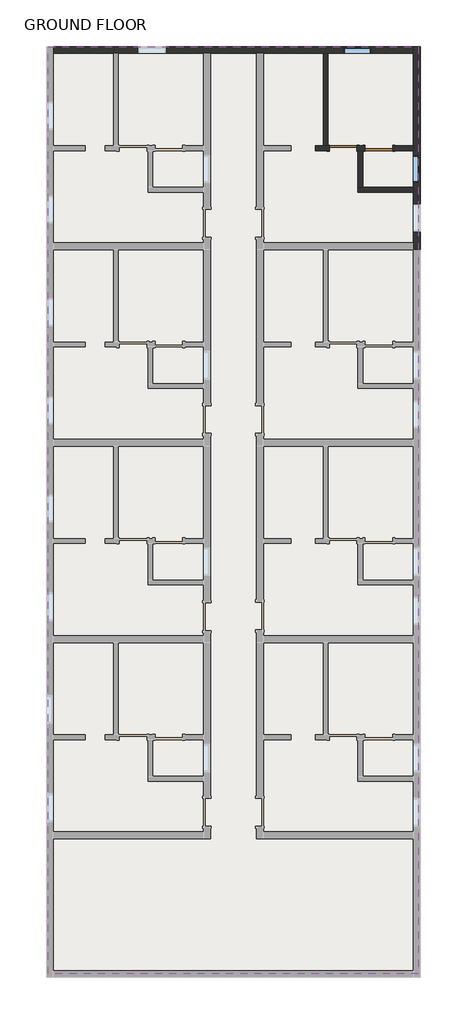
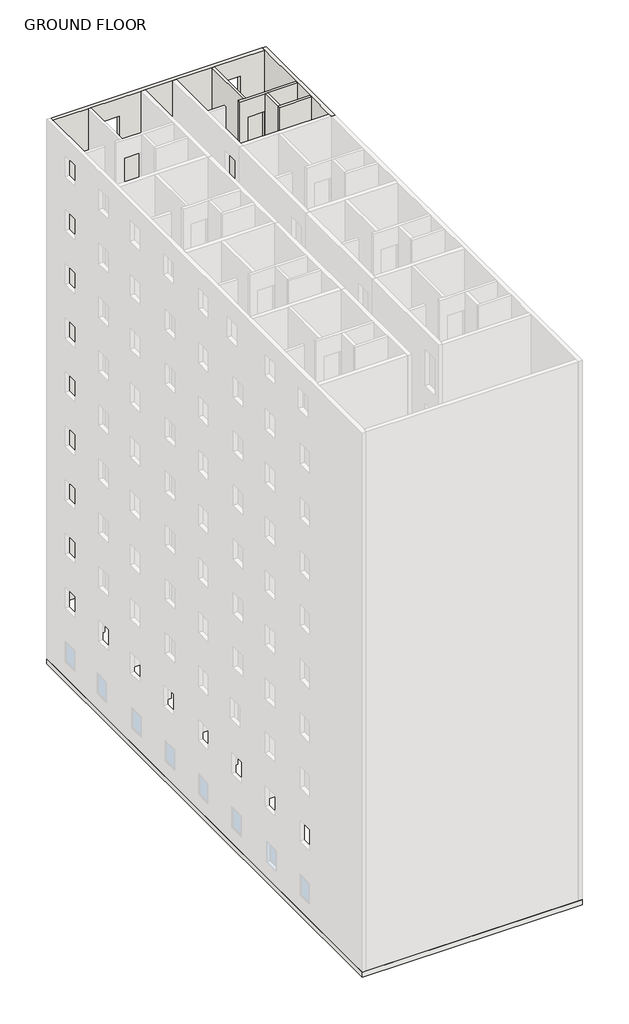
# One storey, part 7 of 7: 6 walls, 3 slabs, 2 doors, 2 windows.
"""IFC4 building model written with IfcOpenShell, lengths in millimetres."""

from ifc_helpers import new_model, si_unit, frame, origin, origin_with_axes, place, context, project, spatial, polyline, outline, extrude, faceted_brep, transform, mapped, element, save
from components import door_686f89d2, door_16372e1c, window_c1f32544

model = new_model("IFC4")

# Units and contexts
model_context = context("Model", 3, world=origin())
ifc_project = project(units=[si_unit("LENGTHUNIT", "METRE", prefix="MILLI")], contexts=[model_context])

# Site, building, storey
site = spatial("IfcSite", under=ifc_project)
building = spatial("IfcBuilding", under=site)
storey = spatial("IfcBuildingStorey", under=building, Name="GROUND FLOOR", Elevation=0.0)

# Doors
placement = place(None, origin())
door_shape = door_686f89d2(model_context)
element("IfcDoor", 1, ObjectType="Single-Flush : 36\" x 84\"", at=placement, inside=storey, context=model_context, shape_type="MappedRepresentation", body=[
    mapped(door_shape, transform((-2929.3902461, 11952.2710592, 0.0), x_axis=(-1.0, 0.0, 0.0), y_axis=(0.0, -1.0, 0.0), z_axis=(0.0, 0.0, 1.0))),
])
door_2_shape = door_16372e1c(model_context)
element("IfcDoor", 2, ObjectType="Single-Flush : 36\" x 84\"", at=placement, inside=storey, context=model_context, shape_type="MappedRepresentation", body=[
    mapped(door_2_shape, transform((-1748.2902461, 11952.2710592, 0.0), x_axis=(-1.0, 0.0, 0.0), y_axis=(0.0, -1.0, 0.0), z_axis=(0.0, 0.0, 1.0))),
])

# Slabs
element("IfcSlab", 3, ObjectType="Generic - 12\"", at=placement, inside=storey, context=model_context, shape_type="SweptSolid", body=[
    extrude(outline(polyline([(-440.1902461, 15305.0710592), (-440.1902461, -15289.2289408), (-12670.2902461, -15289.2289408), (-12670.2902461, 15305.0710592), (-440.1902461, 15305.0710592)])), frame((0.0, 0.0, 3073.4), z_axis=(0.0, 0.0, 1.0), x_axis=(1.0, 0.0, 0.0)), (0.0, 0.0, 1.0), 127.0),
])
element("IfcSlab", 4, ObjectType="Generic - 12\"", at=placement, inside=storey, context=model_context, shape_type="SweptSolid", body=[
    extrude(outline(polyline([(-490.9902461, 15305.0710592), (-490.9902461, -15289.2289408), (-12721.0902461, -15289.2289408), (-12721.0902461, 15305.0710592), (-490.9902461, 15305.0710592)])), frame((0.0, 0.0, -127.0), z_axis=(0.0, 0.0, 1.0), x_axis=(1.0, 0.0, 0.0)), (0.0, 0.0, 1.0), 127.0),
])
element("IfcSlab", 5, ObjectType="Generic - 12\" - Filled", at=placement, inside=storey, context=model_context, shape_type="SweptSolid", body=[
    extrude(outline(polyline([(-376.6902461, 15305.0710592), (-376.6902461, -15403.5289408), (-12721.0902461, -15403.5289408), (-12721.0902461, 15305.0710592), (-376.6902461, 15305.0710592)])), frame((0.0, 0.0, -304.8), z_axis=(0.0, 0.0, 1.0), x_axis=(1.0, 0.0, 0.0)), (0.0, 0.0, 1.0), 304.8),
])

# Walls
element("IfcWall", 6, ObjectType="INNER WALL 2", at=placement, inside=storey, context=model_context, shape_type="Brep", body=[
    faceted_brep([(-2472.1902461, 11876.0710592, 0.0), (-2434.0902461, 11876.0710592, 0.0), (-2281.6902461, 11876.0710592, 0.0), (-2205.4902461, 11876.0710592, 0.0), (-2205.4902461, 11876.0710592, 2133.6), (-1291.0902461, 11876.0710592, 2133.6), (-1291.0902461, 11876.0710592, 0.0), (-605.2902461, 11876.0710592, 0.0), (-605.2902461, 11876.0710592, 32004.0), (-2281.6902461, 11876.0710592, 32004.0), (-2434.0902461, 11876.0710592, 32004.0), (-3843.7902461, 11876.0710592, 32004.0), (-3843.7902461, 11876.0710592, 0.0), (-3386.5902461, 11876.0710592, 0.0), (-3386.5902461, 11876.0710592, 2133.6), (-2472.1902461, 11876.0710592, 2133.6), (-1291.0902461, 11876.0710592, 3200.4), (-2205.4902461, 11876.0710592, 3200.4), (-2205.4902461, 11876.0710592, 5334.0), (-1291.0902461, 11876.0710592, 5334.0), (-2472.1902461, 11876.0710592, 3200.4), (-3386.5902461, 11876.0710592, 3200.4), (-3386.5902461, 11876.0710592, 5334.0), (-2472.1902461, 11876.0710592, 5334.0), (-1291.0902461, 11876.0710592, 6400.8), (-2205.4902461, 11876.0710592, 6400.8), (-2205.4902461, 11876.0710592, 8534.4), (-1291.0902461, 11876.0710592, 8534.4), (-2472.1902461, 11876.0710592, 6400.8), (-3386.5902461, 11876.0710592, 6400.8), (-3386.5902461, 11876.0710592, 8534.4), (-2472.1902461, 11876.0710592, 8534.4), (-2472.1902461, 11876.0710592, 9601.2), (-3386.5902461, 11876.0710592, 9601.2), (-3386.5902461, 11876.0710592, 11734.8), (-2472.1902461, 11876.0710592, 11734.8), (-1291.0902461, 11876.0710592, 9601.2), (-2205.4902461, 11876.0710592, 9601.2), (-2205.4902461, 11876.0710592, 11734.8), (-1291.0902461, 11876.0710592, 11734.8), (-1291.0902461, 11876.0710592, 12801.6), (-2205.4902461, 11876.0710592, 12801.6), (-2205.4902461, 11876.0710592, 14935.2), (-1291.0902461, 11876.0710592, 14935.2), (-2472.1902461, 11876.0710592, 12801.6), (-3386.5902461, 11876.0710592, 12801.6), (-3386.5902461, 11876.0710592, 14935.2), (-2472.1902461, 11876.0710592, 14935.2), (-1291.0902461, 11876.0710592, 16002.0), (-2205.4902461, 11876.0710592, 16002.0), (-2205.4902461, 11876.0710592, 18135.6), (-1291.0902461, 11876.0710592, 18135.6), (-2472.1902461, 11876.0710592, 16002.0), (-3386.5902461, 11876.0710592, 16002.0), (-3386.5902461, 11876.0710592, 18135.6), (-2472.1902461, 11876.0710592, 18135.6), (-1291.0902461, 11876.0710592, 19202.4), (-2205.4902461, 11876.0710592, 19202.4), (-2205.4902461, 11876.0710592, 21336.0), (-1291.0902461, 11876.0710592, 21336.0), (-2472.1902461, 11876.0710592, 19202.4), (-3386.5902461, 11876.0710592, 19202.4), (-3386.5902461, 11876.0710592, 21336.0), (-2472.1902461, 11876.0710592, 21336.0), (-1291.0902461, 11876.0710592, 22402.8), (-2205.4902461, 11876.0710592, 22402.8), (-2205.4902461, 11876.0710592, 24536.4), (-1291.0902461, 11876.0710592, 24536.4), (-2472.1902461, 11876.0710592, 22402.8), (-3386.5902461, 11876.0710592, 22402.8), (-3386.5902461, 11876.0710592, 24536.4), (-2472.1902461, 11876.0710592, 24536.4), (-2472.1902461, 11876.0710592, 25603.2), (-3386.5902461, 11876.0710592, 25603.2), (-3386.5902461, 11876.0710592, 27736.8), (-2472.1902461, 11876.0710592, 27736.8), (-1291.0902461, 11876.0710592, 25603.2), (-2205.4902461, 11876.0710592, 25603.2), (-2205.4902461, 11876.0710592, 27736.8), (-1291.0902461, 11876.0710592, 27736.8), (-2472.1902461, 11876.0710592, 28803.6), (-3386.5902461, 11876.0710592, 28803.6), (-3386.5902461, 11876.0710592, 30937.2), (-2472.1902461, 11876.0710592, 30937.2), (-1291.0902461, 11876.0710592, 28803.6), (-2205.4902461, 11876.0710592, 28803.6), (-2205.4902461, 11876.0710592, 30937.2), (-1291.0902461, 11876.0710592, 30937.2), (-2205.4902461, 12028.4710592, 2133.6), (-2205.4902461, 12028.4710592, 0.0), (-2472.1902461, 12028.4710592, 0.0), (-2472.1902461, 12028.4710592, 2133.6), (-3386.5902461, 12028.4710592, 2133.6), (-3386.5902461, 12028.4710592, 0.0), (-3424.6902461, 12028.4710592, 0.0), (-3577.0902461, 12028.4710592, 0.0), (-3843.7902461, 12028.4710592, 0.0), (-3843.7902461, 12028.4710592, 32004.0), (-3577.0902461, 12028.4710592, 32004.0), (-3424.6902461, 12028.4710592, 32004.0), (-605.2902461, 12028.4710592, 32004.0), (-605.2902461, 12028.4710592, 0.0), (-1291.0902461, 12028.4710592, 0.0), (-1291.0902461, 12028.4710592, 2133.6), (-1291.0902461, 12028.4710592, 3200.4), (-1291.0902461, 12028.4710592, 5334.0), (-2205.4902461, 12028.4710592, 5334.0), (-2205.4902461, 12028.4710592, 3200.4), (-2472.1902461, 12028.4710592, 3200.4), (-2472.1902461, 12028.4710592, 5334.0), (-3386.5902461, 12028.4710592, 5334.0), (-3386.5902461, 12028.4710592, 3200.4), (-1291.0902461, 12028.4710592, 6400.8), (-1291.0902461, 12028.4710592, 8534.4), (-2205.4902461, 12028.4710592, 8534.4), (-2205.4902461, 12028.4710592, 6400.8), (-2472.1902461, 12028.4710592, 6400.8), (-2472.1902461, 12028.4710592, 8534.4), (-3386.5902461, 12028.4710592, 8534.4), (-3386.5902461, 12028.4710592, 6400.8), (-2472.1902461, 12028.4710592, 9601.2), (-2472.1902461, 12028.4710592, 11734.8), (-3386.5902461, 12028.4710592, 11734.8), (-3386.5902461, 12028.4710592, 9601.2), (-1291.0902461, 12028.4710592, 9601.2), (-1291.0902461, 12028.4710592, 11734.8), (-2205.4902461, 12028.4710592, 11734.8), (-2205.4902461, 12028.4710592, 9601.2), (-1291.0902461, 12028.4710592, 12801.6), (-1291.0902461, 12028.4710592, 14935.2), (-2205.4902461, 12028.4710592, 14935.2), (-2205.4902461, 12028.4710592, 12801.6), (-2472.1902461, 12028.4710592, 12801.6), (-2472.1902461, 12028.4710592, 14935.2), (-3386.5902461, 12028.4710592, 14935.2), (-3386.5902461, 12028.4710592, 12801.6), (-1291.0902461, 12028.4710592, 16002.0), (-1291.0902461, 12028.4710592, 18135.6), (-2205.4902461, 12028.4710592, 18135.6), (-2205.4902461, 12028.4710592, 16002.0), (-2472.1902461, 12028.4710592, 16002.0), (-2472.1902461, 12028.4710592, 18135.6), (-3386.5902461, 12028.4710592, 18135.6), (-3386.5902461, 12028.4710592, 16002.0), (-1291.0902461, 12028.4710592, 19202.4), (-1291.0902461, 12028.4710592, 21336.0), (-2205.4902461, 12028.4710592, 21336.0), (-2205.4902461, 12028.4710592, 19202.4), (-2472.1902461, 12028.4710592, 19202.4), (-2472.1902461, 12028.4710592, 21336.0), (-3386.5902461, 12028.4710592, 21336.0), (-3386.5902461, 12028.4710592, 19202.4), (-1291.0902461, 12028.4710592, 22402.8), (-1291.0902461, 12028.4710592, 24536.4), (-2205.4902461, 12028.4710592, 24536.4), (-2205.4902461, 12028.4710592, 22402.8), (-2472.1902461, 12028.4710592, 22402.8), (-2472.1902461, 12028.4710592, 24536.4), (-3386.5902461, 12028.4710592, 24536.4), (-3386.5902461, 12028.4710592, 22402.8), (-2472.1902461, 12028.4710592, 25603.2), (-2472.1902461, 12028.4710592, 27736.8), (-3386.5902461, 12028.4710592, 27736.8), (-3386.5902461, 12028.4710592, 25603.2), (-1291.0902461, 12028.4710592, 25603.2), (-1291.0902461, 12028.4710592, 27736.8), (-2205.4902461, 12028.4710592, 27736.8), (-2205.4902461, 12028.4710592, 25603.2), (-2472.1902461, 12028.4710592, 28803.6), (-2472.1902461, 12028.4710592, 30937.2), (-3386.5902461, 12028.4710592, 30937.2), (-3386.5902461, 12028.4710592, 28803.6), (-1291.0902461, 12028.4710592, 28803.6), (-1291.0902461, 12028.4710592, 30937.2), (-2205.4902461, 12028.4710592, 30937.2), (-2205.4902461, 12028.4710592, 28803.6)], [[[0, 1, 2, 3, 4, 5, 6, 7, 8, 9, 10, 11, 12, 13, 14, 15], [16, 17, 18, 19], [20, 21, 22, 23], [24, 25, 26, 27], [28, 29, 30, 31], [32, 33, 34, 35], [36, 37, 38, 39], [40, 41, 42, 43], [44, 45, 46, 47], [48, 49, 50, 51], [52, 53, 54, 55], [56, 57, 58, 59], [60, 61, 62, 63], [64, 65, 66, 67], [68, 69, 70, 71], [72, 73, 74, 75], [76, 77, 78, 79], [80, 81, 82, 83], [84, 85, 86, 87]], [[88, 89, 90, 91, 92, 93, 94, 95, 96, 97, 98, 99, 100, 101, 102, 103], [104, 105, 106, 107], [108, 109, 110, 111], [112, 113, 114, 115], [116, 117, 118, 119], [120, 121, 122, 123], [124, 125, 126, 127], [128, 129, 130, 131], [132, 133, 134, 135], [136, 137, 138, 139], [140, 141, 142, 143], [144, 145, 146, 147], [148, 149, 150, 151], [152, 153, 154, 155], [156, 157, 158, 159], [160, 161, 162, 163], [164, 165, 166, 167], [168, 169, 170, 171], [172, 173, 174, 175]], [[96, 95, 94, 93, 13, 12]], [[102, 101, 7, 6]], [[90, 89, 3, 2, 1, 0]], [[11, 10, 9, 8, 100, 99, 98, 97]], [[12, 11, 97, 96]], [[8, 7, 101, 100]], [[14, 13, 93, 92]], [[15, 14, 92, 91]], [[0, 15, 91, 90]], [[4, 3, 89, 88]], [[5, 4, 88, 103]], [[6, 5, 103, 102]], [[17, 16, 104, 107]], [[18, 17, 107, 106]], [[19, 18, 106, 105]], [[16, 19, 105, 104]], [[21, 20, 108, 111]], [[22, 21, 111, 110]], [[23, 22, 110, 109]], [[20, 23, 109, 108]], [[25, 24, 112, 115]], [[26, 25, 115, 114]], [[27, 26, 114, 113]], [[24, 27, 113, 112]], [[29, 28, 116, 119]], [[30, 29, 119, 118]], [[31, 30, 118, 117]], [[28, 31, 117, 116]], [[33, 32, 120, 123]], [[34, 33, 123, 122]], [[35, 34, 122, 121]], [[32, 35, 121, 120]], [[37, 36, 124, 127]], [[38, 37, 127, 126]], [[39, 38, 126, 125]], [[36, 39, 125, 124]], [[41, 40, 128, 131]], [[42, 41, 131, 130]], [[43, 42, 130, 129]], [[40, 43, 129, 128]], [[45, 44, 132, 135]], [[46, 45, 135, 134]], [[47, 46, 134, 133]], [[44, 47, 133, 132]], [[49, 48, 136, 139]], [[50, 49, 139, 138]], [[51, 50, 138, 137]], [[48, 51, 137, 136]], [[53, 52, 140, 143]], [[54, 53, 143, 142]], [[55, 54, 142, 141]], [[52, 55, 141, 140]], [[57, 56, 144, 147]], [[58, 57, 147, 146]], [[59, 58, 146, 145]], [[56, 59, 145, 144]], [[61, 60, 148, 151]], [[62, 61, 151, 150]], [[63, 62, 150, 149]], [[60, 63, 149, 148]], [[65, 64, 152, 155]], [[66, 65, 155, 154]], [[67, 66, 154, 153]], [[64, 67, 153, 152]], [[69, 68, 156, 159]], [[70, 69, 159, 158]], [[71, 70, 158, 157]], [[68, 71, 157, 156]], [[73, 72, 160, 163]], [[74, 73, 163, 162]], [[75, 74, 162, 161]], [[72, 75, 161, 160]], [[77, 76, 164, 167]], [[78, 77, 167, 166]], [[79, 78, 166, 165]], [[76, 79, 165, 164]], [[81, 80, 168, 171]], [[82, 81, 171, 170]], [[83, 82, 170, 169]], [[80, 83, 169, 168]], [[85, 84, 172, 175]], [[86, 85, 175, 174]], [[87, 86, 174, 173]], [[84, 87, 173, 172]]]),
])
element("IfcWall", 7, ObjectType="INNER WALL 2", at=placement, inside=storey, context=model_context, shape_type="SweptSolid", body=[
    extrude(outline(polyline([(-3424.6902461, 15076.4710592), (-3424.6902461, 12028.4710592), (-3577.0902461, 12028.4710592), (-3577.0902461, 15076.4710592), (-3424.6902461, 15076.4710592)])), origin_with_axes(), (0.0, 0.0, 1.0), 32004.0),
])
element("IfcWall", 8, ObjectType="INNER WALL 2", at=placement, inside=storey, context=model_context, shape_type="Brep", body=[
    faceted_brep([(-605.2902461, 10656.8710592, 0.0), (-2281.6902461, 10656.8710592, 0.0), (-2434.0902461, 10656.8710592, 0.0), (-2434.0902461, 10656.8710592, 32004.0), (-2281.6902461, 10656.8710592, 32004.0), (-605.2902461, 10656.8710592, 32004.0), (-605.2902461, 10504.4710592, 0.0), (-605.2902461, 10504.4710592, 32004.0), (-2434.0902461, 10504.4710592, 32004.0), (-2434.0902461, 10504.4710592, 0.0)], [[[0, 1, 2, 3, 4, 5]], [[6, 7, 8, 9]], [[2, 1, 0, 6, 9]], [[5, 4, 3, 8, 7]], [[0, 5, 7, 6]], [[3, 2, 9, 8]]]),
])
element("IfcWall", 9, ObjectType="INNER WALL 2", at=placement, inside=storey, context=model_context, shape_type="SweptSolid", body=[
    extrude(outline(polyline([(-2281.6902461, 11876.0710592), (-2281.6902461, 10656.8710592), (-2434.0902461, 10656.8710592), (-2434.0902461, 11876.0710592), (-2281.6902461, 11876.0710592)])), origin_with_axes(), (0.0, 0.0, 1.0), 32004.0),
])
element("IfcWall", 10, ObjectType="OUTER WALL", at=placement, inside=storey, context=model_context, shape_type="Brep", body=[
    faceted_brep([(-376.6902461, 8599.4710592, 0.0), (-376.6902461, 15305.0710592, 0.0), (-376.6902461, 15305.0710592, 32004.0), (-376.6902461, 8599.4710592, 32004.0), (-376.6902461, 9190.0210592, 2133.6), (-376.6902461, 10104.4210592, 2133.6), (-376.6902461, 10104.4210592, 914.4), (-376.6902461, 9190.0210592, 914.4), (-376.6902461, 10809.2710592, 2133.6), (-376.6902461, 11723.6710592, 2133.6), (-376.6902461, 11723.6710592, 914.4), (-376.6902461, 10809.2710592, 914.4), (-376.6902461, 10809.2710592, 5334.0), (-376.6902461, 11723.6710592, 5334.0), (-376.6902461, 11723.6710592, 4114.8), (-376.6902461, 10809.2710592, 4114.8), (-376.6902461, 9190.0210592, 5334.0), (-376.6902461, 10104.4210592, 5334.0), (-376.6902461, 10104.4210592, 4114.8), (-376.6902461, 9190.0210592, 4114.8), (-376.6902461, 10809.2710592, 8534.4), (-376.6902461, 11723.6710592, 8534.4), (-376.6902461, 11723.6710592, 7315.2), (-376.6902461, 10809.2710592, 7315.2), (-376.6902461, 9190.0210592, 8534.4), (-376.6902461, 10104.4210592, 8534.4), (-376.6902461, 10104.4210592, 7315.2), (-376.6902461, 9190.0210592, 7315.2), (-376.6902461, 9190.0210592, 11734.8), (-376.6902461, 10104.4210592, 11734.8), (-376.6902461, 10104.4210592, 10515.6), (-376.6902461, 9190.0210592, 10515.6), (-376.6902461, 10809.2710592, 11734.8), (-376.6902461, 11723.6710592, 11734.8), (-376.6902461, 11723.6710592, 10515.6), (-376.6902461, 10809.2710592, 10515.6), (-376.6902461, 10809.2710592, 14935.2), (-376.6902461, 11723.6710592, 14935.2), (-376.6902461, 11723.6710592, 13716.0), (-376.6902461, 10809.2710592, 13716.0), (-376.6902461, 9190.0210592, 14935.2), (-376.6902461, 10104.4210592, 14935.2), (-376.6902461, 10104.4210592, 13716.0), (-376.6902461, 9190.0210592, 13716.0), (-376.6902461, 10809.2710592, 18135.6), (-376.6902461, 11723.6710592, 18135.6), (-376.6902461, 11723.6710592, 16916.4), (-376.6902461, 10809.2710592, 16916.4), (-376.6902461, 9190.0210592, 18135.6), (-376.6902461, 10104.4210592, 18135.6), (-376.6902461, 10104.4210592, 16916.4), (-376.6902461, 9190.0210592, 16916.4), (-376.6902461, 10809.2710592, 21336.0), (-376.6902461, 11723.6710592, 21336.0), (-376.6902461, 11723.6710592, 20116.8), (-376.6902461, 10809.2710592, 20116.8), (-376.6902461, 9190.0210592, 21336.0), (-376.6902461, 10104.4210592, 21336.0), (-376.6902461, 10104.4210592, 20116.8), (-376.6902461, 9190.0210592, 20116.8), (-376.6902461, 10809.2710592, 24536.4), (-376.6902461, 11723.6710592, 24536.4), (-376.6902461, 11723.6710592, 23317.2), (-376.6902461, 10809.2710592, 23317.2), (-376.6902461, 9190.0210592, 24536.4), (-376.6902461, 10104.4210592, 24536.4), (-376.6902461, 10104.4210592, 23317.2), (-376.6902461, 9190.0210592, 23317.2), (-376.6902461, 10809.2710592, 27736.8), (-376.6902461, 11723.6710592, 27736.8), (-376.6902461, 11723.6710592, 26517.6), (-376.6902461, 10809.2710592, 26517.6), (-376.6902461, 9190.0210592, 27736.8), (-376.6902461, 10104.4210592, 27736.8), (-376.6902461, 10104.4210592, 26517.6), (-376.6902461, 9190.0210592, 26517.6), (-376.6902461, 10809.2710592, 30937.2), (-376.6902461, 11723.6710592, 30937.2), (-376.6902461, 11723.6710592, 29718.0), (-376.6902461, 10809.2710592, 29718.0), (-376.6902461, 9190.0210592, 30937.2), (-376.6902461, 10104.4210592, 30937.2), (-376.6902461, 10104.4210592, 29718.0), (-376.6902461, 9190.0210592, 29718.0), (-605.2902461, 8599.4710592, 0.0), (-605.2902461, 8599.4710592, 32004.0), (-605.2902461, 8828.0710592, 32004.0), (-605.2902461, 10504.4710592, 32004.0), (-605.2902461, 10656.8710592, 32004.0), (-605.2902461, 11876.0710592, 32004.0), (-605.2902461, 12028.4710592, 32004.0), (-605.2902461, 15076.4710592, 32004.0), (-605.2902461, 15305.0710592, 32004.0), (-605.2902461, 15305.0710592, 0.0), (-605.2902461, 15076.4710592, 0.0), (-605.2902461, 12028.4710592, 0.0), (-605.2902461, 11876.0710592, 0.0), (-605.2902461, 10656.8710592, 0.0), (-605.2902461, 10504.4710592, 0.0), (-605.2902461, 8828.0710592, 0.0), (-605.2902461, 9190.0210592, 2133.6), (-605.2902461, 9190.0210592, 914.4), (-605.2902461, 10104.4210592, 914.4), (-605.2902461, 10104.4210592, 2133.6), (-605.2902461, 10809.2710592, 2133.6), (-605.2902461, 10809.2710592, 914.4), (-605.2902461, 11723.6710592, 914.4), (-605.2902461, 11723.6710592, 2133.6), (-605.2902461, 10809.2710592, 5334.0), (-605.2902461, 10809.2710592, 4114.8), (-605.2902461, 11723.6710592, 4114.8), (-605.2902461, 11723.6710592, 5334.0), (-605.2902461, 9190.0210592, 5334.0), (-605.2902461, 9190.0210592, 4114.8), (-605.2902461, 10104.4210592, 4114.8), (-605.2902461, 10104.4210592, 5334.0), (-605.2902461, 10809.2710592, 8534.4), (-605.2902461, 10809.2710592, 7315.2), (-605.2902461, 11723.6710592, 7315.2), (-605.2902461, 11723.6710592, 8534.4), (-605.2902461, 9190.0210592, 8534.4), (-605.2902461, 9190.0210592, 7315.2), (-605.2902461, 10104.4210592, 7315.2), (-605.2902461, 10104.4210592, 8534.4), (-605.2902461, 9190.0210592, 11734.8), (-605.2902461, 9190.0210592, 10515.6), (-605.2902461, 10104.4210592, 10515.6), (-605.2902461, 10104.4210592, 11734.8), (-605.2902461, 10809.2710592, 11734.8), (-605.2902461, 10809.2710592, 10515.6), (-605.2902461, 11723.6710592, 10515.6), (-605.2902461, 11723.6710592, 11734.8), (-605.2902461, 10809.2710592, 14935.2), (-605.2902461, 10809.2710592, 13716.0), (-605.2902461, 11723.6710592, 13716.0), (-605.2902461, 11723.6710592, 14935.2), (-605.2902461, 9190.0210592, 14935.2), (-605.2902461, 9190.0210592, 13716.0), (-605.2902461, 10104.4210592, 13716.0), (-605.2902461, 10104.4210592, 14935.2), (-605.2902461, 10809.2710592, 18135.6), (-605.2902461, 10809.2710592, 16916.4), (-605.2902461, 11723.6710592, 16916.4), (-605.2902461, 11723.6710592, 18135.6), (-605.2902461, 9190.0210592, 18135.6), (-605.2902461, 9190.0210592, 16916.4), (-605.2902461, 10104.4210592, 16916.4), (-605.2902461, 10104.4210592, 18135.6), (-605.2902461, 10809.2710592, 21336.0), (-605.2902461, 10809.2710592, 20116.8), (-605.2902461, 11723.6710592, 20116.8), (-605.2902461, 11723.6710592, 21336.0), (-605.2902461, 9190.0210592, 21336.0), (-605.2902461, 9190.0210592, 20116.8), (-605.2902461, 10104.4210592, 20116.8), (-605.2902461, 10104.4210592, 21336.0), (-605.2902461, 10809.2710592, 24536.4), (-605.2902461, 10809.2710592, 23317.2), (-605.2902461, 11723.6710592, 23317.2), (-605.2902461, 11723.6710592, 24536.4), (-605.2902461, 9190.0210592, 24536.4), (-605.2902461, 9190.0210592, 23317.2), (-605.2902461, 10104.4210592, 23317.2), (-605.2902461, 10104.4210592, 24536.4), (-605.2902461, 10809.2710592, 27736.8), (-605.2902461, 10809.2710592, 26517.6), (-605.2902461, 11723.6710592, 26517.6), (-605.2902461, 11723.6710592, 27736.8), (-605.2902461, 9190.0210592, 27736.8), (-605.2902461, 9190.0210592, 26517.6), (-605.2902461, 10104.4210592, 26517.6), (-605.2902461, 10104.4210592, 27736.8), (-605.2902461, 10809.2710592, 30937.2), (-605.2902461, 10809.2710592, 29718.0), (-605.2902461, 11723.6710592, 29718.0), (-605.2902461, 11723.6710592, 30937.2), (-605.2902461, 9190.0210592, 30937.2), (-605.2902461, 9190.0210592, 29718.0), (-605.2902461, 10104.4210592, 29718.0), (-605.2902461, 10104.4210592, 30937.2)], [[[0, 1, 2, 3], [4, 5, 6, 7], [8, 9, 10, 11], [12, 13, 14, 15], [16, 17, 18, 19], [20, 21, 22, 23], [24, 25, 26, 27], [28, 29, 30, 31], [32, 33, 34, 35], [36, 37, 38, 39], [40, 41, 42, 43], [44, 45, 46, 47], [48, 49, 50, 51], [52, 53, 54, 55], [56, 57, 58, 59], [60, 61, 62, 63], [64, 65, 66, 67], [68, 69, 70, 71], [72, 73, 74, 75], [76, 77, 78, 79], [80, 81, 82, 83]], [[84, 85, 86, 87, 88, 89, 90, 91, 92, 93, 94, 95, 96, 97, 98, 99], [100, 101, 102, 103], [104, 105, 106, 107], [108, 109, 110, 111], [112, 113, 114, 115], [116, 117, 118, 119], [120, 121, 122, 123], [124, 125, 126, 127], [128, 129, 130, 131], [132, 133, 134, 135], [136, 137, 138, 139], [140, 141, 142, 143], [144, 145, 146, 147], [148, 149, 150, 151], [152, 153, 154, 155], [156, 157, 158, 159], [160, 161, 162, 163], [164, 165, 166, 167], [168, 169, 170, 171], [172, 173, 174, 175], [176, 177, 178, 179]], [[1, 0, 84, 99, 98, 97, 96, 95, 94, 93]], [[3, 2, 92, 91, 90, 89, 88, 87, 86, 85]], [[0, 3, 85, 84]], [[101, 100, 4, 7]], [[102, 101, 7, 6]], [[103, 102, 6, 5]], [[100, 103, 5, 4]], [[105, 104, 8, 11]], [[106, 105, 11, 10]], [[107, 106, 10, 9]], [[104, 107, 9, 8]], [[2, 1, 93, 92]], [[109, 108, 12, 15]], [[110, 109, 15, 14]], [[111, 110, 14, 13]], [[108, 111, 13, 12]], [[113, 112, 16, 19]], [[114, 113, 19, 18]], [[115, 114, 18, 17]], [[112, 115, 17, 16]], [[117, 116, 20, 23]], [[118, 117, 23, 22]], [[119, 118, 22, 21]], [[116, 119, 21, 20]], [[121, 120, 24, 27]], [[122, 121, 27, 26]], [[123, 122, 26, 25]], [[120, 123, 25, 24]], [[125, 124, 28, 31]], [[126, 125, 31, 30]], [[127, 126, 30, 29]], [[124, 127, 29, 28]], [[129, 128, 32, 35]], [[130, 129, 35, 34]], [[131, 130, 34, 33]], [[128, 131, 33, 32]], [[133, 132, 36, 39]], [[134, 133, 39, 38]], [[135, 134, 38, 37]], [[132, 135, 37, 36]], [[137, 136, 40, 43]], [[138, 137, 43, 42]], [[139, 138, 42, 41]], [[136, 139, 41, 40]], [[141, 140, 44, 47]], [[142, 141, 47, 46]], [[143, 142, 46, 45]], [[140, 143, 45, 44]], [[145, 144, 48, 51]], [[146, 145, 51, 50]], [[147, 146, 50, 49]], [[144, 147, 49, 48]], [[149, 148, 52, 55]], [[150, 149, 55, 54]], [[151, 150, 54, 53]], [[148, 151, 53, 52]], [[153, 152, 56, 59]], [[154, 153, 59, 58]], [[155, 154, 58, 57]], [[152, 155, 57, 56]], [[157, 156, 60, 63]], [[158, 157, 63, 62]], [[159, 158, 62, 61]], [[156, 159, 61, 60]], [[161, 160, 64, 67]], [[162, 161, 67, 66]], [[163, 162, 66, 65]], [[160, 163, 65, 64]], [[165, 164, 68, 71]], [[166, 165, 71, 70]], [[167, 166, 70, 69]], [[164, 167, 69, 68]], [[169, 168, 72, 75]], [[170, 169, 75, 74]], [[171, 170, 74, 73]], [[168, 171, 73, 72]], [[173, 172, 76, 79]], [[174, 173, 79, 78]], [[175, 174, 78, 77]], [[172, 175, 77, 76]], [[177, 176, 80, 83]], [[178, 177, 83, 82]], [[179, 178, 82, 81]], [[176, 179, 81, 80]]]),
])
element("IfcWall", 11, ObjectType="OUTER WALL", at=placement, inside=storey, context=model_context, shape_type="Brep", body=[
    faceted_brep([(-12492.4902461, 15076.4710592, 0.0), (-10511.2902461, 15076.4710592, 0.0), (-10358.8902461, 15076.4710592, 0.0), (-7539.4902461, 15076.4710592, 0.0), (-7310.8902461, 15076.4710592, 0.0), (-5786.8902461, 15076.4710592, 0.0), (-5558.2902461, 15076.4710592, 0.0), (-3577.0902461, 15076.4710592, 0.0), (-3424.6902461, 15076.4710592, 0.0), (-605.2902461, 15076.4710592, 0.0), (-605.2902461, 15076.4710592, 32004.0), (-3424.6902461, 15076.4710592, 32004.0), (-3577.0902461, 15076.4710592, 32004.0), (-5558.2902461, 15076.4710592, 32004.0), (-5786.8902461, 15076.4710592, 32004.0), (-7310.8902461, 15076.4710592, 32004.0), (-7539.4902461, 15076.4710592, 32004.0), (-10358.8902461, 15076.4710592, 32004.0), (-10511.2902461, 15076.4710592, 32004.0), (-12492.4902461, 15076.4710592, 32004.0), (-1976.8902461, 15076.4710592, 5334.0), (-1976.8902461, 15076.4710592, 4114.8), (-2891.2902461, 15076.4710592, 4114.8), (-2891.2902461, 15076.4710592, 5334.0), (-8758.6902461, 15076.4710592, 5334.0), (-8758.6902461, 15076.4710592, 4114.8), (-9673.0902461, 15076.4710592, 4114.8), (-9673.0902461, 15076.4710592, 5334.0), (-8758.6902461, 15076.4710592, 8534.4), (-8758.6902461, 15076.4710592, 7315.2), (-9673.0902461, 15076.4710592, 7315.2), (-9673.0902461, 15076.4710592, 8534.4), (-1976.8902461, 15076.4710592, 8534.4), (-1976.8902461, 15076.4710592, 7315.2), (-2891.2902461, 15076.4710592, 7315.2), (-2891.2902461, 15076.4710592, 8534.4), (-1976.8902461, 15076.4710592, 11734.8), (-1976.8902461, 15076.4710592, 10515.6), (-2891.2902461, 15076.4710592, 10515.6), (-2891.2902461, 15076.4710592, 11734.8), (-8758.6902461, 15076.4710592, 11734.8), (-8758.6902461, 15076.4710592, 10515.6), (-9673.0902461, 15076.4710592, 10515.6), (-9673.0902461, 15076.4710592, 11734.8), (-8758.6902461, 15076.4710592, 14935.2), (-8758.6902461, 15076.4710592, 13716.0), (-9673.0902461, 15076.4710592, 13716.0), (-9673.0902461, 15076.4710592, 14935.2), (-1976.8902461, 15076.4710592, 14935.2), (-1976.8902461, 15076.4710592, 13716.0), (-2891.2902461, 15076.4710592, 13716.0), (-2891.2902461, 15076.4710592, 14935.2), (-8777.7402461, 15076.4710592, 2133.6), (-8777.7402461, 15076.4710592, 914.4), (-9692.1402461, 15076.4710592, 914.4), (-9692.1402461, 15076.4710592, 2133.6), (-1995.9402461, 15076.4710592, 2133.6), (-1995.9402461, 15076.4710592, 914.4), (-2910.3402461, 15076.4710592, 914.4), (-2910.3402461, 15076.4710592, 2133.6), (-8758.6902461, 15076.4710592, 18135.6), (-8758.6902461, 15076.4710592, 16916.4), (-9673.0902461, 15076.4710592, 16916.4), (-9673.0902461, 15076.4710592, 18135.6), (-1976.8902461, 15076.4710592, 18135.6), (-1976.8902461, 15076.4710592, 16916.4), (-2891.2902461, 15076.4710592, 16916.4), (-2891.2902461, 15076.4710592, 18135.6), (-8758.6902461, 15076.4710592, 21336.0), (-8758.6902461, 15076.4710592, 20116.8), (-9673.0902461, 15076.4710592, 20116.8), (-9673.0902461, 15076.4710592, 21336.0), (-1976.8902461, 15076.4710592, 21336.0), (-1976.8902461, 15076.4710592, 20116.8), (-2891.2902461, 15076.4710592, 20116.8), (-2891.2902461, 15076.4710592, 21336.0), (-8758.6902461, 15076.4710592, 24536.4), (-8758.6902461, 15076.4710592, 23317.2), (-9673.0902461, 15076.4710592, 23317.2), (-9673.0902461, 15076.4710592, 24536.4), (-1976.8902461, 15076.4710592, 24536.4), (-1976.8902461, 15076.4710592, 23317.2), (-2891.2902461, 15076.4710592, 23317.2), (-2891.2902461, 15076.4710592, 24536.4), (-8758.6902461, 15076.4710592, 27736.8), (-8758.6902461, 15076.4710592, 26517.6), (-9673.0902461, 15076.4710592, 26517.6), (-9673.0902461, 15076.4710592, 27736.8), (-1976.8902461, 15076.4710592, 27736.8), (-1976.8902461, 15076.4710592, 26517.6), (-2891.2902461, 15076.4710592, 26517.6), (-2891.2902461, 15076.4710592, 27736.8), (-8758.6902461, 15076.4710592, 30937.2), (-8758.6902461, 15076.4710592, 29718.0), (-9673.0902461, 15076.4710592, 29718.0), (-9673.0902461, 15076.4710592, 30937.2), (-1976.8902461, 15076.4710592, 30937.2), (-1976.8902461, 15076.4710592, 29718.0), (-2891.2902461, 15076.4710592, 29718.0), (-2891.2902461, 15076.4710592, 30937.2), (-12492.4902461, 15305.0710592, 0.0), (-12492.4902461, 15305.0710592, 32004.0), (-605.2902461, 15305.0710592, 32004.0), (-605.2902461, 15305.0710592, 0.0), (-1976.8902461, 15305.0710592, 5334.0), (-2891.2902461, 15305.0710592, 5334.0), (-2891.2902461, 15305.0710592, 4114.8), (-1976.8902461, 15305.0710592, 4114.8), (-8758.6902461, 15305.0710592, 5334.0), (-9673.0902461, 15305.0710592, 5334.0), (-9673.0902461, 15305.0710592, 4114.8), (-8758.6902461, 15305.0710592, 4114.8), (-8758.6902461, 15305.0710592, 8534.4), (-9673.0902461, 15305.0710592, 8534.4), (-9673.0902461, 15305.0710592, 7315.2), (-8758.6902461, 15305.0710592, 7315.2), (-1976.8902461, 15305.0710592, 8534.4), (-2891.2902461, 15305.0710592, 8534.4), (-2891.2902461, 15305.0710592, 7315.2), (-1976.8902461, 15305.0710592, 7315.2), (-1976.8902461, 15305.0710592, 11734.8), (-2891.2902461, 15305.0710592, 11734.8), (-2891.2902461, 15305.0710592, 10515.6), (-1976.8902461, 15305.0710592, 10515.6), (-8758.6902461, 15305.0710592, 11734.8), (-9673.0902461, 15305.0710592, 11734.8), (-9673.0902461, 15305.0710592, 10515.6), (-8758.6902461, 15305.0710592, 10515.6), (-8758.6902461, 15305.0710592, 14935.2), (-9673.0902461, 15305.0710592, 14935.2), (-9673.0902461, 15305.0710592, 13716.0), (-8758.6902461, 15305.0710592, 13716.0), (-1976.8902461, 15305.0710592, 14935.2), (-2891.2902461, 15305.0710592, 14935.2), (-2891.2902461, 15305.0710592, 13716.0), (-1976.8902461, 15305.0710592, 13716.0), (-8777.7402461, 15305.0710592, 2133.6), (-9692.1402461, 15305.0710592, 2133.6), (-9692.1402461, 15305.0710592, 914.4), (-8777.7402461, 15305.0710592, 914.4), (-1995.9402461, 15305.0710592, 2133.6), (-2910.3402461, 15305.0710592, 2133.6), (-2910.3402461, 15305.0710592, 914.4), (-1995.9402461, 15305.0710592, 914.4), (-8758.6902461, 15305.0710592, 18135.6), (-9673.0902461, 15305.0710592, 18135.6), (-9673.0902461, 15305.0710592, 16916.4), (-8758.6902461, 15305.0710592, 16916.4), (-1976.8902461, 15305.0710592, 18135.6), (-2891.2902461, 15305.0710592, 18135.6), (-2891.2902461, 15305.0710592, 16916.4), (-1976.8902461, 15305.0710592, 16916.4), (-8758.6902461, 15305.0710592, 21336.0), (-9673.0902461, 15305.0710592, 21336.0), (-9673.0902461, 15305.0710592, 20116.8), (-8758.6902461, 15305.0710592, 20116.8), (-1976.8902461, 15305.0710592, 21336.0), (-2891.2902461, 15305.0710592, 21336.0), (-2891.2902461, 15305.0710592, 20116.8), (-1976.8902461, 15305.0710592, 20116.8), (-8758.6902461, 15305.0710592, 24536.4), (-9673.0902461, 15305.0710592, 24536.4), (-9673.0902461, 15305.0710592, 23317.2), (-8758.6902461, 15305.0710592, 23317.2), (-1976.8902461, 15305.0710592, 24536.4), (-2891.2902461, 15305.0710592, 24536.4), (-2891.2902461, 15305.0710592, 23317.2), (-1976.8902461, 15305.0710592, 23317.2), (-8758.6902461, 15305.0710592, 27736.8), (-9673.0902461, 15305.0710592, 27736.8), (-9673.0902461, 15305.0710592, 26517.6), (-8758.6902461, 15305.0710592, 26517.6), (-1976.8902461, 15305.0710592, 27736.8), (-2891.2902461, 15305.0710592, 27736.8), (-2891.2902461, 15305.0710592, 26517.6), (-1976.8902461, 15305.0710592, 26517.6), (-8758.6902461, 15305.0710592, 30937.2), (-9673.0902461, 15305.0710592, 30937.2), (-9673.0902461, 15305.0710592, 29718.0), (-8758.6902461, 15305.0710592, 29718.0), (-1976.8902461, 15305.0710592, 30937.2), (-2891.2902461, 15305.0710592, 30937.2), (-2891.2902461, 15305.0710592, 29718.0), (-1976.8902461, 15305.0710592, 29718.0)], [[[0, 1, 2, 3, 4, 5, 6, 7, 8, 9, 10, 11, 12, 13, 14, 15, 16, 17, 18, 19], [20, 21, 22, 23], [24, 25, 26, 27], [28, 29, 30, 31], [32, 33, 34, 35], [36, 37, 38, 39], [40, 41, 42, 43], [44, 45, 46, 47], [48, 49, 50, 51], [52, 53, 54, 55], [56, 57, 58, 59], [60, 61, 62, 63], [64, 65, 66, 67], [68, 69, 70, 71], [72, 73, 74, 75], [76, 77, 78, 79], [80, 81, 82, 83], [84, 85, 86, 87], [88, 89, 90, 91], [92, 93, 94, 95], [96, 97, 98, 99]], [[100, 101, 102, 103], [104, 105, 106, 107], [108, 109, 110, 111], [112, 113, 114, 115], [116, 117, 118, 119], [120, 121, 122, 123], [124, 125, 126, 127], [128, 129, 130, 131], [132, 133, 134, 135], [136, 137, 138, 139], [140, 141, 142, 143], [144, 145, 146, 147], [148, 149, 150, 151], [152, 153, 154, 155], [156, 157, 158, 159], [160, 161, 162, 163], [164, 165, 166, 167], [168, 169, 170, 171], [172, 173, 174, 175], [176, 177, 178, 179], [180, 181, 182, 183]], [[9, 8, 7, 6, 5, 4, 3, 2, 1, 0, 100, 103]], [[19, 18, 17, 16, 15, 14, 13, 12, 11, 10, 102, 101]], [[0, 19, 101, 100]], [[10, 9, 103, 102]], [[21, 20, 104, 107]], [[22, 21, 107, 106]], [[23, 22, 106, 105]], [[20, 23, 105, 104]], [[25, 24, 108, 111]], [[26, 25, 111, 110]], [[27, 26, 110, 109]], [[24, 27, 109, 108]], [[29, 28, 112, 115]], [[30, 29, 115, 114]], [[31, 30, 114, 113]], [[28, 31, 113, 112]], [[33, 32, 116, 119]], [[34, 33, 119, 118]], [[35, 34, 118, 117]], [[32, 35, 117, 116]], [[37, 36, 120, 123]], [[38, 37, 123, 122]], [[39, 38, 122, 121]], [[36, 39, 121, 120]], [[41, 40, 124, 127]], [[42, 41, 127, 126]], [[43, 42, 126, 125]], [[40, 43, 125, 124]], [[45, 44, 128, 131]], [[46, 45, 131, 130]], [[47, 46, 130, 129]], [[44, 47, 129, 128]], [[49, 48, 132, 135]], [[50, 49, 135, 134]], [[51, 50, 134, 133]], [[48, 51, 133, 132]], [[53, 52, 136, 139]], [[54, 53, 139, 138]], [[55, 54, 138, 137]], [[52, 55, 137, 136]], [[57, 56, 140, 143]], [[58, 57, 143, 142]], [[59, 58, 142, 141]], [[56, 59, 141, 140]], [[61, 60, 144, 147]], [[62, 61, 147, 146]], [[63, 62, 146, 145]], [[60, 63, 145, 144]], [[65, 64, 148, 151]], [[66, 65, 151, 150]], [[67, 66, 150, 149]], [[64, 67, 149, 148]], [[69, 68, 152, 155]], [[70, 69, 155, 154]], [[71, 70, 154, 153]], [[68, 71, 153, 152]], [[73, 72, 156, 159]], [[74, 73, 159, 158]], [[75, 74, 158, 157]], [[72, 75, 157, 156]], [[77, 76, 160, 163]], [[78, 77, 163, 162]], [[79, 78, 162, 161]], [[76, 79, 161, 160]], [[81, 80, 164, 167]], [[82, 81, 167, 166]], [[83, 82, 166, 165]], [[80, 83, 165, 164]], [[85, 84, 168, 171]], [[86, 85, 171, 170]], [[87, 86, 170, 169]], [[84, 87, 169, 168]], [[89, 88, 172, 175]], [[90, 89, 175, 174]], [[91, 90, 174, 173]], [[88, 91, 173, 172]], [[93, 92, 176, 179]], [[94, 93, 179, 178]], [[95, 94, 178, 177]], [[92, 95, 177, 176]], [[97, 96, 180, 183]], [[98, 97, 183, 182]], [[99, 98, 182, 181]], [[96, 99, 181, 180]]]),
])

# Windows
window_shape = window_c1f32544(model_context)
element("IfcWindow", 12, ObjectType="Fixed : 36\" x 48\"", at=placement, inside=storey, context=model_context, shape_type="MappedRepresentation", body=[
    mapped(window_shape, transform((-490.9902461, 11228.3710592, 0.0), x_axis=(0.0, -1.0, 0.0), y_axis=(1.0, 0.0, 0.0), z_axis=(0.0, 0.0, 1.0))),
])
element("IfcWindow", 13, ObjectType="Fixed : 36\" x 48\"", at=placement, inside=storey, context=model_context, shape_type="MappedRepresentation", body=[
    mapped(window_shape, transform((-2415.0402461, 15190.7710592, 0.0), x_axis=(1.0, 0.0, 0.0), y_axis=(0.0, 1.0, 0.0), z_axis=(0.0, 0.0, 1.0))),
])

save(model, "model.ifc")

# Revit data of these elements
# Type "Single-Flush : 36\" x 84\""
#   Type Mark = "1"
#   Construction Type Id = "MDOOR"
#   Assembly Code = "C1020"
#   Analytic Construction = "Metal"
#   Thickness = 0' - 2"
#   Heat Transfer Coefficient (U) = 0.651978 BTU/(h·ft²·°F)
#   Height = 7' - 0"
#   Trim Projection Ext = 0' - 1"
#   Trim Projection Int = 0' - 1"
#   Trim Width = 0' - 3"
#   Width = 3' - 0"
#   Define Thermal Properties by = 1
#   Door Material = Door - Panel
#   Frame Material = Door - Frame
#   Visual Light Transmittance = 0
#   Solar Heat Gain Coefficient = 0
#   Function = (empty or 0)
#   Wall Closure = (empty or 0)
# Type "Generic - 12\""
#   Assembly Code = "B1010"
#   Function = 0
#   Layers, outside or top first: 0' - 5" no material (function 1)
# Type "Generic - 12\" - Filled"
#   Assembly Code = "B1010"
#   Function = 0
#   Layers, outside or top first: 1' - 0" no material (function 1)
# Type "INNER WALL 2"
#   Assembly Code = "B2010"
#   Layers, outside or top first: 0' - 6" no material (function 1)
# Type "OUTER WALL"
#   Assembly Code = "B2010"
#   Layers, outside or top first: 0' - 9" no material (function 1)
# Type "Fixed : 36\" x 48\""
#   Type Mark = "1"
#   Construction Type Id = "GSP4R"
#   Assembly Code = "B2020100"
#   Analytic Construction = "1/8 in Pilkington single glazing"
#   Visual Light Transmittance = 0.9
#   Solar Heat Gain Coefficient = 0.78
#   Heat Transfer Coefficient (U) = 0.6496 BTU/(h·ft²·°F)
#   Height = 4' - 0"
#   Default Sill Height = 3' - 0"
#   Width = 3' - 0"
#   Window Inset = 0' - 0 3/4"
#   Define Thermal Properties by = 1
#   Glass Pane Material = Glass
#   Sash Material = Sash
#   Wall Closure = (empty or 0)
# Elements 1, 2 (IfcDoor, "Single-Flush : 36\" x 84\"")
#   Phase Created = New Construction
#   Materials on its faces: "Door - Frame", "Door - Panel"
# Element 3 (IfcSlab, "Generic - 12\"")
#   Height Offset From Level = 10' - 6"
#   Phase Created = New Construction
#   Materials on its faces: "Default Floor"
# Element 4 (IfcSlab, "Generic - 12\"")
#   Height Offset From Level = 0' - 0"
#   Phase Created = New Construction
#   Materials on its faces: "Default Floor"
# Element 5 (IfcSlab, "Generic - 12\" - Filled")
#   Height Offset From Level = 0' - 0"
#   Phase Created = New Construction
#   Materials on its faces: "Default Floor"
# Elements 6, 7, 8, 9 (IfcWall, "INNER WALL 2")
#   Top Offset = 0' - 0"
#   Base Offset = 0' - 0"
#   Unconnected Height = 105' - 0"
#   wall height = 105' - 0"
#   Phase Created = New Construction
#   Base Constraint = GROUND FLOOR
#   Materials on its faces: "Default Wall"
# Elements 10, 11 (IfcWall, "OUTER WALL")
#   Top Offset = 0' - 0"
#   Base Offset = 0' - 0"
#   Unconnected Height = 105' - 0"
#   wall height = 105' - 0"
#   Phase Created = New Construction
#   Base Constraint = GROUND FLOOR
#   Materials on its faces: "Default Wall"
# Element 12 (IfcWindow, "Fixed : 36\" x 48\"")
#   Mark = "18"
#   Phase Created = New Construction
#   Materials on its faces: "Sash", "Glass"
# Element 13 (IfcWindow, "Fixed : 36\" x 48\"")
#   Mark = "116"
#   Phase Created = New Construction
#   Materials on its faces: "Sash", "Glass"
# Materials
#   "Door - Panel": class "Wood", colour RGB 210 159 95, transparency 0
#   "Door - Frame": colour RGB 118 70 51, transparency 0
#   "Glass": class "Glass", colour RGB 0 128 192, transparency 0.75, Description = "Soda Lime Glass", Cost = 0
#   "Sash": class "Wood", colour RGB 224 178 126, transparency 0
#   "Default Floor": colour RGB 128 128 128, transparency 0
#   "Default Wall": colour RGB 128 128 128, transparency 0
